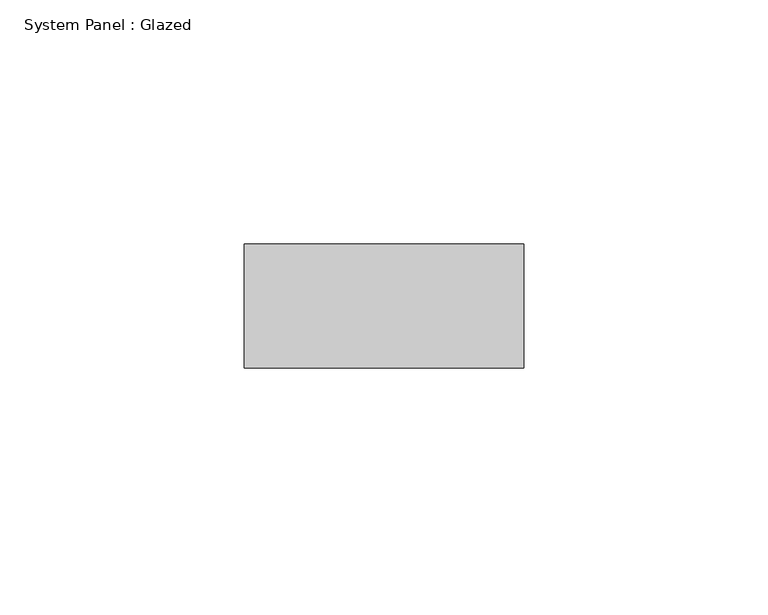
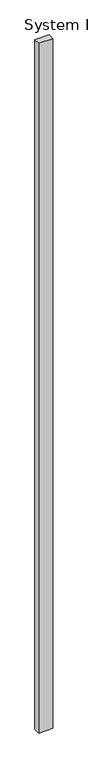
"""IFC4 building model written with IfcOpenShell, lengths in millimetres: plate geometry, System Panel : Glazed."""

from ifc_helpers import new_model, si_unit, origin, origin_with_axes, place, context, project, spatial, polyline, outline, extrude, source, transform, mapped, element, save


def system_panel_glazed_e7b2b8ad(model_context):
    return source(origin(), model_context, "Body", "SweptSolid", [
        extrude(outline(polyline([(28.575, -44.45), (-28.575, -44.45), (-28.575, -19.05), (28.575, -19.05), (28.575, -44.45)])), origin_with_axes(), (0.0, 0.0, 1.0), 2921.0),
    ])


if __name__ == "__main__":
    model = new_model("IFC4")
    model_context = context("Model", 3, world=origin())
    ifc_project = project(units=[si_unit("LENGTHUNIT", "METRE", prefix="MILLI")], contexts=[model_context])
    site = spatial("IfcSite", under=ifc_project)
    building = spatial("IfcBuilding", under=site)
    placement = place(None, origin())
    system_panel_glazed_shape = system_panel_glazed_e7b2b8ad(model_context)
    element("IfcPlate", 1, ObjectType="System Panel : Glazed", at=placement, inside=building, context=model_context, shape_type="MappedRepresentation", body=[
        mapped(system_panel_glazed_shape, transform((0.0, 0.0, 0.0), x_axis=(1.0, 0.0, 0.0), y_axis=(0.0, 1.0, 0.0), z_axis=(0.0, 0.0, 1.0))),
    ])
    save(model, "model.ifc")

# Revit data of these elements
# Type "System Panel : Glazed"
#   Construction Type Id = "GSP4R"
#   Analytic Construction = "1/8 in Pilkington single glazing"
#   Visual Light Transmittance = 0.9
#   Solar Heat Gain Coefficient = 0.86
#   Heat Transfer Coefficient (U) = 1.18115 BTU/(h·ft²·°F)
# Element 1 (IfcPlate, "System Panel : Glazed")
#   Materials on its faces: "Glass"
# Materials
#   "Glass": class "Glass", colour RGB 0 128 192, transparency 0.75, Description = "Soda Lime Glass", Cost = 0
